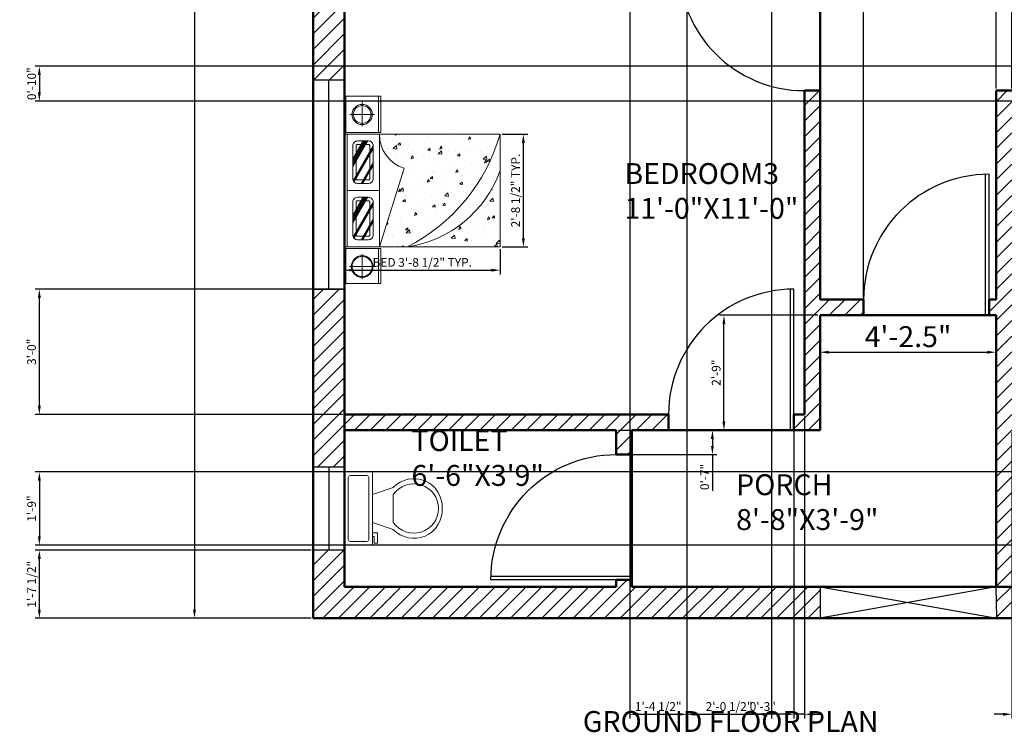
# Model space of a CAD drawing. Units: inches. Extents: x 3064 to 3516, y 2736 to 3280.
# Tile 1 of 5: x 3064 to 3346, y 2736 to 2941. Entities that reach past the tile are written whole.
import ezdxf

# ---------------------------------------------------------------- set-up
doc = ezdxf.new("R2010")
doc.units = ezdxf.units.IN
for name, color, linetype, lineweight in [('A-ANNO-DIMS', 2, 'Continuous', 18), ('A-ANNO-TEXT', 7, 'Continuous', 25), ('A-AREA-IDEN', 6, 'Continuous', 25), ('A-DOOR', 3, 'Continuous', 25), ('A-FLOR-ENTR', 1, 'Continuous', 25), ('A-FLOR-FIXT', 9, 'Continuous', 20), ('A-FURN', 8, 'Continuous', 18), ('A-FURN-PATT', 9, 'Continuous', 13), ('A-GLAZ', 5, 'Continuous', 25), ('A-WALL', 7, 'Continuous', 50), ('A-WALL-PATT', 8, 'Continuous', 13)]:
    doc.layers.add(name, color=color, linetype=linetype, lineweight=lineweight)
doc.styles.get("Standard").update_dxf_attribs({"font": 'arial.ttf'})
doc.dimstyles.new('ISO-25', dxfattribs={"dimtxt": 2.5, "dimasz": 2.5, "dimexe": 1.25, "dimexo": 0.625, "dimtad": 1, "dimlunit": 3, "dimtxsty": 'Standard', "dimcen": 2.5, "dimadec": 0, "dimazin": 0, "dimtfac": 1, "dimtmove": 0, "dimatfit": 3, "dimfxl": 1, "dimarcsym": 0})

# ---------------------------------------------------------------- blocks, each defined once
blk = doc.blocks.new('*D2')
at = {"layer": 'A-ANNO-DIMS', "color": 0, "lineweight": -2, "transparency": 16777216}
for p, q in [((3293.4, 2848.4), (3293.4, 2844.15)), ((3343.9, 2848.4), (3343.9, 2844.15)), ((3295.9, 2845.4), (3341.4, 2845.4))]:
    blk.add_line(p, q, dxfattribs=at)
at = {"layer": 'A-ANNO-DIMS', "color": 0, "transparency": 16777216}
for points in [[(3295.9, 2845.82), (3295.9, 2844.98), (3293.4, 2845.4)], [(3341.4, 2845.82), (3341.4, 2844.98), (3343.9, 2845.4)]]:
    blk.add_solid(points, dxfattribs=at)
at = {"layer": 'Defpoints', "color": 0, "transparency": 16777216}
for p in [(3293.4, 2849.02), (3343.9, 2849.02), (3343.9, 2845.4)]:
    blk.add_point(p, dxfattribs=at)
at = {"layer": 'A-ANNO-DIMS', "color": 0, "transparency": 16777216, "insert": (3318.65, 2849.09), "char_height": 6, "attachment_point": 5}
blk.add_mtext('4\'-2.5"', dxfattribs=at)
blk = doc.blocks.new('*D4')
at = {"layer": 'A-ANNO-DIMS', "color": 0, "lineweight": -2, "transparency": 16777216}
for p, q in [((3147.27, 3211.51), (3112.57, 3211.51)), ((3113.82, 3209.01), (3113.82, 2771.51)), ((3147.27, 2769.01), (3112.57, 2769.01))]:
    blk.add_line(p, q, dxfattribs=at)
at = {"layer": 'A-ANNO-DIMS', "color": 0, "transparency": 16777216}
for points in [[(3113.4, 3209.01), (3114.23, 3209.01), (3113.82, 3211.51)], [(3113.4, 2771.51), (3114.23, 2771.51), (3113.82, 2769.01)]]:
    blk.add_solid(points, dxfattribs=at)
at = {"layer": 'Defpoints', "color": 0, "transparency": 16777216}
for p in [(3147.9, 3211.51), (3113.82, 2769.01), (3147.9, 2769.01)]:
    blk.add_point(p, dxfattribs=at)
at = {"layer": 'A-ANNO-DIMS', "color": 0, "transparency": 16777216, "insert": (3110.13, 2990.26), "char_height": 6, "attachment_point": 5, "rotation": 90}
blk.add_mtext('36\'-10.5"', dxfattribs=at)
blk = doc.blocks.new('*U6')
for p, q in [((9.5, -6), (9.5, -2)), ((-8, -8.5), (-8, -8)), ((-7, -8), (-7, -9.5)), ((-4, -8), (-6, -14)), ((4, -8), (6, -14)), ((-10, -8.5), (-8, -8.5)), ((-10, -9.5), (-10, -8.5)), ((-7, -9.5), (-10, -9.5)), ((4, -14), (-4, -14))]:
    blk.add_line(p, q)
blk.add_lwpolyline([(10.5, -8), (10.5, 0), (-10.5, 0), (-10.5, -8)], close=True)
for points in [[(-9.5, -2), (-9.5, -6)], [(8.5, -1), (-8.5, -1)], [(-8.5, -7), (8.5, -7)]]:
    blk.add_lwpolyline(points)
for centre, radius, start, end in [((-8.625, -1.875), 0.8839, 81.8699, 188.1301), ((8.625, -1.875), 0.8839, 351.8699, 98.1301), ((-8.625, -6.125), 0.8839, 171.869898, 278.1301), ((8.625, -6.125), 0.8839, 261.8699, 8.1301), ((-0.4772, -19.9188), 8.0953, 133.01722, 273.38), ((0.0374, -19.8731), 7.127, 124.50543, 269.7), ((-0.0373, -19.8731), 7.127, 270.3, 55.4946), ((0.4773, -19.9188), 8.0953, 266.62, 46.9828)]:
    blk.add_arc(centre, radius, start, end)
blk = doc.blocks.new('DOOR-SWING-36IN')
for p, q in [((-1, -4.5), (-1, 36)), ((0, 0), (0, 36))]:
    blk.add_line(p, q)
blk.add_arc((0, 0), 36, 90, 180)
blk = doc.blocks.new('WIN-60IN')
for p, q in [((0, 60), (0, 0)), ((9, 60), (0, 60)), ((4.5, 60), (4.5, 0)), ((9, 0), (9, 60)), ((0, 0), (9, 0))]:
    blk.add_line(p, q)
blk = doc.blocks.new('WIN-24IN')
for p, q in [((0, 24), (9, 24)), ((0, 0), (0, 24)), ((4.5, 24), (4.5, 0)), ((9, 24), (9, 0)), ((9, 0), (0, 0))]:
    blk.add_line(p, q)
blk = doc.blocks.new('BEDSIDE-TABLE-A')
for p, q in [((0, 0), (0, 10.49)), ((0, 10.49), (10.04, 10.49)), ((4.67, 1.81), (4.67, 8.9)), ((9.38, 0), (9.38, 10.49)), ((10.04, 10.49), (10.04, 0)), ((1.1, 5.18), (8.23, 5.18)), ((10.04, 0), (0, 0))]:
    blk.add_line(p, q)
for radius in [2.89, 2.54]:
    blk.add_circle((4.67, 5.18), radius)
blk = doc.blocks.new('BEDSIDE-TABLE-B')
for p, q in [((10.04, 10.04), (0, 10.04)), ((0, 10.04), (0, 0)), ((9.34, 0), (9.34, 10.04)), ((10.04, 0), (10.04, 10.04)), ((4.67, 1.21), (4.67, 8.43)), ((1.04, 4.86), (8.55, 4.86)), ((0, 0), (10.04, 0))]:
    blk.add_line(p, q)
for radius in [3.11, 2.89]:
    blk.add_circle((4.67, 4.86), radius)
blk = doc.blocks.new('BED-FRAME-AND-COVER')
for p, q in [((0, 32.36), (44.63, 32.36)), ((0, 0), (0, 32.36)), ((0.73, 0), (0.73, 32.36)), ((10.02, 0), (10.02, 32.36)), ((44.63, 32.36), (44.63, 0)), ((10.02, 0), (17.09, 22.61)), ((10.02, 16.18), (0.73, 16.18)), ((44.63, 0), (0, 0))]:
    blk.add_line(p, q)
for centre, radius, start, end in [((20, 32.16), 9.98, 178.8468, 253.0453), ((-5.57, 46.57), 52.17, 296.7955, 344.1914), ((13.16, 33.03), 33.38, 278.2583, 340.5572)]:
    blk.add_arc(centre, radius, start, end)
blk = doc.blocks.new('*D29')
at = {"layer": 'A-ANNO-DIMS', "color": 0, "lineweight": -2, "transparency": 16777216}
for p, q in [((3156.9, 2875.02), (3156.9, 2867.7)), ((3201.53, 2875.02), (3201.53, 2867.7)), ((3159.4, 2868.95), (3199.03, 2868.95))]:
    blk.add_line(p, q, dxfattribs=at)
at = {"layer": 'A-ANNO-DIMS', "color": 0, "transparency": 16777216}
for points in [[(3159.4, 2869.37), (3159.4, 2868.54), (3156.9, 2868.95)], [(3199.03, 2869.37), (3199.03, 2868.54), (3201.53, 2868.95)]]:
    blk.add_solid(points, dxfattribs=at)
at = {"layer": 'Defpoints', "color": 0, "transparency": 16777216}
for p in [(3156.9, 2875.65), (3201.53, 2875.65), (3201.53, 2868.95)]:
    blk.add_point(p, dxfattribs=at)
at = {"layer": 'A-ANNO-DIMS', "color": 0, "transparency": 16777216, "insert": (3179.21, 2870.87), "char_height": 2.5, "attachment_point": 5}
blk.add_mtext('BED 3\'-8 1/2" TYP.', dxfattribs=at)
blk = doc.blocks.new('*D30')
at = {"layer": 'A-ANNO-DIMS', "color": 0, "lineweight": -2, "transparency": 16777216}
for p, q in [((3202.15, 2908.01), (3209.47, 2908.01)), ((3208.22, 2878.15), (3208.22, 2905.51)), ((3202.15, 2875.65), (3209.47, 2875.65))]:
    blk.add_line(p, q, dxfattribs=at)
at = {"layer": 'A-ANNO-DIMS', "color": 0, "transparency": 16777216}
for points in [[(3207.81, 2905.51), (3208.64, 2905.51), (3208.22, 2908.01)], [(3207.81, 2878.15), (3208.64, 2878.15), (3208.22, 2875.65)]]:
    blk.add_solid(points, dxfattribs=at)
at = {"layer": 'Defpoints', "color": 0, "transparency": 16777216}
for p in [(3201.53, 2908.01), (3208.22, 2908.01), (3201.53, 2875.65)]:
    blk.add_point(p, dxfattribs=at)
at = {"layer": 'A-ANNO-DIMS', "color": 0, "transparency": 16777216, "insert": (3206.31, 2891.83), "char_height": 2.5, "attachment_point": 5, "rotation": 90}
blk.add_mtext('2\'-8 1/2" TYP.', dxfattribs=at)
blk = doc.blocks.new('*D37')
at = {"layer": 'A-ANNO-DIMS', "color": 0, "lineweight": -2, "transparency": 16777216}
for p, q in [((3147.27, 2788.51), (3068.05, 2788.51)), ((3069.3, 2771.51), (3069.3, 2786.01)), ((3147.27, 2769.01), (3068.05, 2769.01))]:
    blk.add_line(p, q, dxfattribs=at)
at = {"layer": 'A-ANNO-DIMS', "color": 0, "transparency": 16777216}
for points in [[(3068.88, 2786.01), (3069.71, 2786.01), (3069.3, 2788.51)], [(3068.88, 2771.51), (3069.71, 2771.51), (3069.3, 2769.01)]]:
    blk.add_solid(points, dxfattribs=at)
at = {"layer": 'Defpoints', "color": 0, "transparency": 16777216}
for p in [(3069.3, 2788.51), (3147.9, 2788.51), (3147.9, 2769.01)]:
    blk.add_point(p, dxfattribs=at)
at = {"layer": 'A-ANNO-DIMS', "color": 0, "transparency": 16777216, "insert": (3067.38, 2778.76), "char_height": 2.5, "attachment_point": 5, "rotation": 90}
blk.add_mtext('1\'-7 1/2"', dxfattribs=at)
blk = doc.blocks.new('*D38')
at = {"layer": 'A-ANNO-DIMS', "color": 0, "lineweight": -2, "transparency": 16777216}
for p, q in [((3156.27, 2863.51), (3068.05, 2863.51)), ((3069.3, 2830.01), (3069.3, 2861.01)), ((3156.27, 2827.51), (3068.05, 2827.51))]:
    blk.add_line(p, q, dxfattribs=at)
at = {"layer": 'A-ANNO-DIMS', "color": 0, "transparency": 16777216}
for points in [[(3068.88, 2861.01), (3069.71, 2861.01), (3069.3, 2863.51)], [(3068.88, 2830.01), (3069.71, 2830.01), (3069.3, 2827.51)]]:
    blk.add_solid(points, dxfattribs=at)
at = {"layer": 'Defpoints', "color": 0, "transparency": 16777216}
for p in [(3069.3, 2863.51), (3156.9, 2863.51), (3156.9, 2827.51)]:
    blk.add_point(p, dxfattribs=at)
at = {"layer": 'A-ANNO-DIMS', "color": 0, "transparency": 16777216, "insert": (3067.39, 2845.51), "char_height": 2.5, "attachment_point": 5, "rotation": 90}
blk.add_mtext('3\'-0"', dxfattribs=at)
blk = doc.blocks.new('*D44')
at = {"layer": 'A-ANNO-DIMS', "color": 0, "lineweight": -2, "transparency": 16777216}
for p, q in [((3341.4, 3239.11), (3325.18, 3239.11)), ((3343.9, 2921.14), (3343.9, 3240.36)), ((3348.4, 3239.11), (3343.9, 3239.11)), ((3348.4, 2921.14), (3348.4, 3240.36)), ((3350.9, 3239.11), (3353.4, 3239.11))]:
    blk.add_line(p, q, dxfattribs=at)
at = {"layer": 'A-ANNO-DIMS', "color": 0, "transparency": 16777216}
for points in [[(3341.4, 3239.53), (3341.4, 3238.7), (3343.9, 3239.11)], [(3350.9, 3239.53), (3350.9, 3238.7), (3348.4, 3239.11)]]:
    blk.add_solid(points, dxfattribs=at)
at = {"layer": 'Defpoints', "color": 0, "transparency": 16777216}
for p in [(3343.9, 3239.11), (3343.9, 2920.51), (3348.4, 2920.51)]:
    blk.add_point(p, dxfattribs=at)
at = {"layer": 'A-ANNO-DIMS', "color": 0, "transparency": 16777216, "insert": (3332.04, 3241.03), "char_height": 2.5, "attachment_point": 5}
blk.add_mtext('0\'-4 1/2"', dxfattribs=at)
blk = doc.blocks.new('*D45')
at = {"layer": 'A-ANNO-DIMS', "color": 0, "lineweight": -2, "transparency": 16777216}
for p, q in [((3386.77, 2927.51), (3068.05, 2927.51)), ((3069.3, 2925.01), (3069.3, 2920.01)), ((3386.77, 2917.51), (3068.05, 2917.51))]:
    blk.add_line(p, q, dxfattribs=at)
at = {"layer": 'A-ANNO-DIMS', "color": 0, "transparency": 16777216}
for points in [[(3068.88, 2925.01), (3069.71, 2925.01), (3069.3, 2927.51)], [(3068.88, 2920.01), (3069.71, 2920.01), (3069.3, 2917.51)]]:
    blk.add_solid(points, dxfattribs=at)
at = {"layer": 'Defpoints', "color": 0, "transparency": 16777216}
for p in [(3387.4, 2927.51), (3069.3, 2917.51), (3387.4, 2917.51)]:
    blk.add_point(p, dxfattribs=at)
at = {"layer": 'A-ANNO-DIMS', "color": 0, "transparency": 16777216, "insert": (3067.4, 2922.51), "char_height": 2.5, "attachment_point": 5, "rotation": 90}
blk.add_mtext('0\'-10"', dxfattribs=at)
blk = doc.blocks.new('*D47')
at = {"layer": 'A-ANNO-DIMS', "color": 0, "lineweight": -2, "transparency": 16777216}
for p, q in [((3292.77, 2856.01), (3264.55, 2856.01)), ((3265.8, 2825.51), (3265.8, 2853.51)), ((3292.77, 2823.01), (3264.55, 2823.01))]:
    blk.add_line(p, q, dxfattribs=at)
at = {"layer": 'A-ANNO-DIMS', "color": 0, "transparency": 16777216}
for points in [[(3265.38, 2853.51), (3266.21, 2853.51), (3265.8, 2856.01)], [(3265.38, 2825.51), (3266.21, 2825.51), (3265.8, 2823.01)]]:
    blk.add_solid(points, dxfattribs=at)
at = {"layer": 'Defpoints', "color": 0, "transparency": 16777216}
for p in [(3265.8, 2856.01), (3293.4, 2856.01), (3293.4, 2823.01)]:
    blk.add_point(p, dxfattribs=at)
at = {"layer": 'A-ANNO-DIMS', "color": 0, "transparency": 16777216, "insert": (3263.9, 2839.51), "char_height": 2.5, "attachment_point": 5, "rotation": 90}
blk.add_mtext('2\'-9"', dxfattribs=at)
blk = doc.blocks.new('*D48')
at = {"layer": 'A-ANNO-DIMS', "color": 0, "lineweight": -2, "transparency": 16777216}
for p, q in [((3417.77, 2811.01), (3068.05, 2811.01)), ((3069.3, 2808.51), (3069.3, 2792.51)), ((3417.77, 2790.01), (3068.05, 2790.01))]:
    blk.add_line(p, q, dxfattribs=at)
at = {"layer": 'A-ANNO-DIMS', "color": 0, "transparency": 16777216}
for points in [[(3068.88, 2808.51), (3069.71, 2808.51), (3069.3, 2811.01)], [(3068.88, 2792.51), (3069.71, 2792.51), (3069.3, 2790.01)]]:
    blk.add_solid(points, dxfattribs=at)
at = {"layer": 'Defpoints', "color": 0, "transparency": 16777216}
for p in [(3418.4, 2811.01), (3069.3, 2790.01), (3418.4, 2790.01)]:
    blk.add_point(p, dxfattribs=at)
at = {"layer": 'A-ANNO-DIMS', "color": 0, "transparency": 16777216, "insert": (3067.4, 2800.51), "char_height": 2.5, "attachment_point": 5, "rotation": 90}
blk.add_mtext('1\'-9"', dxfattribs=at)
blk = doc.blocks.new('*D53')
at = {"layer": 'A-ANNO-DIMS', "color": 0, "lineweight": -2, "transparency": 16777216}
for p, q in [((3238.74, 2963.39), (3238.74, 2740.16)), ((3255.12, 2963.39), (3255.12, 2740.16)), ((3241.24, 2741.41), (3252.62, 2741.41))]:
    blk.add_line(p, q, dxfattribs=at)
at = {"layer": 'A-ANNO-DIMS', "color": 0, "transparency": 16777216}
for points in [[(3241.24, 2741.83), (3241.24, 2741), (3238.74, 2741.41)], [(3252.62, 2741.83), (3252.62, 2741), (3255.12, 2741.41)]]:
    blk.add_solid(points, dxfattribs=at)
at = {"layer": 'Defpoints', "color": 0, "transparency": 16777216}
for p in [(3238.74, 2964.01), (3255.12, 2964.01), (3255.12, 2741.41)]:
    blk.add_point(p, dxfattribs=at)
at = {"layer": 'A-ANNO-DIMS', "color": 0, "transparency": 16777216, "insert": (3246.93, 2743.33), "char_height": 2.5, "attachment_point": 5}
blk.add_mtext('1\'-4 1/2"', dxfattribs=at)
blk = doc.blocks.new('*D54')
at = {"layer": 'A-ANNO-DIMS', "color": 0, "lineweight": -2, "transparency": 16777216}
for p, q in [((3255.12, 2963.39), (3255.12, 2740.16)), ((3279.41, 2963.39), (3279.41, 2740.16)), ((3257.62, 2741.41), (3276.91, 2741.41))]:
    blk.add_line(p, q, dxfattribs=at)
at = {"layer": 'A-ANNO-DIMS', "color": 0, "transparency": 16777216}
for points in [[(3257.62, 2741.83), (3257.62, 2741), (3255.12, 2741.41)], [(3276.91, 2741.83), (3276.91, 2741), (3279.41, 2741.41)]]:
    blk.add_solid(points, dxfattribs=at)
at = {"layer": 'Defpoints', "color": 0, "transparency": 16777216}
for p in [(3255.12, 2964.01), (3279.41, 2964.01), (3279.41, 2741.41)]:
    blk.add_point(p, dxfattribs=at)
at = {"layer": 'A-ANNO-DIMS', "color": 0, "transparency": 16777216, "insert": (3267.26, 2743.33), "char_height": 2.5, "attachment_point": 5}
blk.add_mtext('2\'-0 1/2"', dxfattribs=at)
blk = doc.blocks.new('*D58')
at = {"layer": 'A-ANNO-DIMS', "color": 0, "lineweight": -2, "transparency": 16777216}
for p, q in [((3235.52, 2823.01), (3263.75, 2823.01)), ((3262.5, 2820.51), (3262.5, 2818.51)), ((3235.52, 2816.01), (3263.75, 2816.01)), ((3262.5, 2816.01), (3262.5, 2805.62))]:
    blk.add_line(p, q, dxfattribs=at)
at = {"layer": 'A-ANNO-DIMS', "color": 0, "transparency": 16777216}
for points in [[(3262.08, 2820.51), (3262.91, 2820.51), (3262.5, 2823.01)], [(3262.08, 2818.51), (3262.91, 2818.51), (3262.5, 2816.01)]]:
    blk.add_solid(points, dxfattribs=at)
at = {"layer": 'Defpoints', "color": 0, "transparency": 16777216}
for p in [(3234.9, 2823.01), (3234.9, 2816.01), (3262.5, 2816.01)]:
    blk.add_point(p, dxfattribs=at)
at = {"layer": 'A-ANNO-DIMS', "color": 0, "transparency": 16777216, "insert": (3260.6, 2809.57), "char_height": 2.5, "attachment_point": 5, "rotation": 90}
blk.add_mtext('0\'-7"', dxfattribs=at)
blk = doc.blocks.new('*D60')
at = {"layer": 'A-ANNO-DIMS', "color": 0, "lineweight": -2, "transparency": 16777216}
for p, q in [((3285.9, 2826.89), (3285.9, 2740.16)), ((3288.9, 2826.89), (3288.9, 2740.16)), ((3283.4, 2741.41), (3273, 2741.41)), ((3288.9, 2741.41), (3285.9, 2741.41)), ((3291.4, 2741.41), (3293.9, 2741.41))]:
    blk.add_line(p, q, dxfattribs=at)
at = {"layer": 'A-ANNO-DIMS', "color": 0, "transparency": 16777216}
for points in [[(3283.4, 2741.83), (3283.4, 2741), (3285.9, 2741.41)], [(3291.4, 2741.83), (3291.4, 2741), (3288.9, 2741.41)]]:
    blk.add_solid(points, dxfattribs=at)
at = {"layer": 'Defpoints', "color": 0, "transparency": 16777216}
for p in [(3285.9, 2827.51), (3288.9, 2827.51), (3285.9, 2741.41)]:
    blk.add_point(p, dxfattribs=at)
at = {"layer": 'A-ANNO-DIMS', "color": 0, "transparency": 16777216, "insert": (3276.95, 2743.32), "char_height": 2.5, "attachment_point": 5}
blk.add_mtext('0\'-3"', dxfattribs=at)
blk = doc.blocks.new('*D61')
at = {"layer": 'A-ANNO-DIMS', "color": 0, "lineweight": -2, "transparency": 16777216}
for p, q in [((3293.4, 2861.14), (3293.4, 3240.36)), ((3295.9, 3239.11), (3303.4, 3239.11)), ((3305.9, 2861.14), (3305.9, 3240.36)), ((3305.9, 3239.11), (3321.88, 3239.11))]:
    blk.add_line(p, q, dxfattribs=at)
at = {"layer": 'A-ANNO-DIMS', "color": 0, "transparency": 16777216}
for points in [[(3295.9, 3239.53), (3295.9, 3238.7), (3293.4, 3239.11)], [(3303.4, 3239.53), (3303.4, 3238.7), (3305.9, 3239.11)]]:
    blk.add_solid(points, dxfattribs=at)
at = {"layer": 'Defpoints', "color": 0, "transparency": 16777216}
for p in [(3305.9, 3239.11), (3293.4, 2860.51), (3305.9, 2860.51)]:
    blk.add_point(p, dxfattribs=at)
at = {"layer": 'A-ANNO-DIMS', "color": 0, "transparency": 16777216, "insert": (3315.14, 3241.03), "char_height": 2.5, "attachment_point": 5}
blk.add_mtext('1\'-0 1/2"', dxfattribs=at)
blk = doc.blocks.new('*D63')
at = {"layer": 'A-ANNO-DIMS', "color": 0, "lineweight": -2, "transparency": 16777216}
for p, q in [((3348.4, 2822.39), (3348.4, 2740.16)), ((3350.4, 2822.39), (3350.4, 2740.16)), ((3345.9, 2741.41), (3343.4, 2741.41)), ((3348.4, 2741.41), (3350.4, 2741.41)), ((3352.9, 2741.41), (3363.29, 2741.41))]:
    blk.add_line(p, q, dxfattribs=at)
at = {"layer": 'A-ANNO-DIMS', "color": 0, "transparency": 16777216}
for points in [[(3345.9, 2741.83), (3345.9, 2741), (3348.4, 2741.41)], [(3352.9, 2741.83), (3352.9, 2741), (3350.4, 2741.41)]]:
    blk.add_solid(points, dxfattribs=at)
at = {"layer": 'Defpoints', "color": 0, "transparency": 16777216}
for p in [(3348.4, 2823.01), (3350.4, 2823.01), (3350.4, 2741.41)]:
    blk.add_point(p, dxfattribs=at)
at = {"layer": 'A-ANNO-DIMS', "color": 0, "transparency": 16777216, "insert": (3359.35, 2743.32), "char_height": 2.5, "attachment_point": 5}
blk.add_mtext('0\'-2"', dxfattribs=at)

msp = doc.modelspace()

# ---------------------------------------------------------------- hatches: boundary and pattern name
at = {"layer": 'A-FURN-PATT'}
h = msp.add_hatch(dxfattribs=at)
h.set_pattern_fill('ANSI31', color=256, scale=0.070287317, angle=15.041628, style=0)
h.paths.add_polyline_path([(3159.249, 2898.533), (3159.249, 2898.613), (3159.249, 2899.06), (3159.249, 2899.507), (3159.249, 2899.587), (3162.981, 2906.063), (3163.028, 2906.063), (3163.285, 2906.063), (3163.543, 2906.063), (3163.589, 2906.063)])
h = msp.add_hatch(dxfattribs=at)
h.set_pattern_fill('ANSI31', color=256, scale=0.070284384, angle=15.041628, style=0)
h.paths.add_polyline_path([(3159.249, 2899.981), (3159.249, 2900.062), (3159.249, 2900.508), (3159.249, 2900.955), (3159.249, 2901.036), (3162.147, 2906.063), (3162.193, 2906.063), (3162.451, 2906.063), (3162.708, 2906.063), (3162.754, 2906.063)])
h = msp.add_hatch(dxfattribs=at)
h.set_pattern_fill('AR-CONC', color=256, scale=0.044631, angle=450, style=0)
h.set_pattern_definition([(220, (5689.692, 3289.2617), (0.711375, -8.131058), [0.850218, -9.352396]), (275, (5689.692, 3289.262), (-8.527021, 1.572917), [0.680174, -7.481917]), (169.549, (5689.7516, 3288.584), (-7.815608, -6.55817), [0.722574, -7.94831]), (223.8158, (5687.425, 3289.262), (1.876385, -12.09849), [1.275327, -14.028594]), (173.3644, (5687.581, 3288.253), (-11.042814, -10.595554), [1.08386, -11.922464]), (278.816, (5687.425, 3289.262), (-11.042795, -10.59557), [1.02026, -11.222875]), (249, (5687.992, 3288.128), (4.564198, -6.766702), [0.850218, -9.352396]), (304, (5687.992, 3288.128), (-8.220467, -2.758277), [0.680174, -7.481917]), (198.5486, (5688.372, 3287.564), (-3.656287, -9.52496), [0.722574, -7.94831]), (232.5, (5689.6923, 3289.2617), (-3.7737637, -0.137847), [0, -7.391227, 0, -7.595279, 0, -7.510257]), (262.5, (5689.6923, 3289.2617), (-4.471145, -2.982219), [0, -4.330443, 0, -7.221183, 0, -2.8624]), (302.5, (5689.6923, 3291.7896), (0.2556787, -6.0515243), [0, -2.834059, 0, -8.842265, 0, -11.733006]), (312.5, (5689.6923, 3292.9233), (-1.134806, -6.611132), [0, -3.684277, 0, -5.872171, 0, -8.332134])])
edge = h.paths.add_edge_path()
edge.add_ellipse((3176.893, 2907.806), major_axis=(7.055, 7.055), ratio=1, start_angle=136.15316, end_angle=208.04534, ccw=False)
edge.add_line((3166.918, 2907.605), (3166.918, 2908.007))
edge.add_line((3166.918, 2908.007), (3201.528, 2908.007))
edge.add_ellipse((3151.329, 2922.22), major_axis=(36.892, 36.892), ratio=1, start_angle=251.7955, end_angle=299.1914, ccw=False)
edge.add_line((3174.849, 2875.649), (3166.918, 2875.649))
edge.add_line((3166.918, 2875.649), (3173.983, 2898.262))
edge = h.paths.add_edge_path()
edge.add_line((3201.528, 2897.57), (3201.528, 2875.649))
edge.add_line((3201.528, 2875.649), (3174.849, 2875.649))
edge.add_ellipse((3170.054, 2908.68), major_axis=(23.601, -23.601), ratio=1, start_angle=323.25827, end_angle=385.55722)
h = msp.add_hatch(dxfattribs=at)
h.set_pattern_fill('ANSI31', color=256, scale=0.070289157, angle=15.041628, style=0)
h.paths.add_polyline_path([(3159.656, 2894.255), (3159.629, 2894.288), (3159.478, 2894.474), (3159.353, 2894.704), (3159.331, 2894.746), (3165.137, 2904.819), (3165.137, 2904.738), (3165.137, 2904.291), (3165.137, 2903.845), (3165.137, 2903.764)])
h = msp.add_hatch(dxfattribs=at)
h.set_pattern_fill('ANSI31', color=256, scale=0.070287466, angle=15.041628, style=0)
h.paths.add_polyline_path([(3162.239, 2893.884), (3162.193, 2893.884), (3161.935, 2893.884), (3161.678, 2893.884), (3161.631, 2893.884), (3165.137, 2899.965), (3165.137, 2899.885), (3165.137, 2899.438), (3165.137, 2898.991), (3165.137, 2898.911)])
h = msp.add_hatch(dxfattribs=at)
h.set_pattern_fill('ANSI31', color=256, scale=0.070289772, angle=15.041628, style=0)
h.paths.add_polyline_path([(3159.249, 2882.354), (3159.249, 2882.435), (3159.249, 2882.881), (3159.249, 2883.328), (3159.249, 2883.409), (3162.981, 2889.884), (3163.028, 2889.884), (3163.285, 2889.884), (3163.543, 2889.884), (3163.589, 2889.884)])
h = msp.add_hatch(dxfattribs=at)
h.set_pattern_fill('ANSI31', color=256, scale=0.070286859, angle=15.041628, style=0)
h.paths.add_polyline_path([(3159.249, 2883.802), (3159.249, 2883.883), (3159.249, 2884.33), (3159.249, 2884.777), (3159.249, 2884.857), (3162.147, 2889.884), (3162.193, 2889.884), (3162.451, 2889.884), (3162.708, 2889.884), (3162.754, 2889.884)])
h = msp.add_hatch(dxfattribs=at)
h.set_pattern_fill('ANSI31', color=256, scale=0.070279531, angle=15.041628, style=0)
h.paths.add_polyline_path([(3159.656, 2878.076), (3159.629, 2878.11), (3159.478, 2878.295), (3159.353, 2878.526), (3159.331, 2878.567), (3165.137, 2888.64), (3165.137, 2888.559), (3165.137, 2888.113), (3165.137, 2887.666), (3165.137, 2887.585)])
h = msp.add_hatch(dxfattribs=at)
h.set_pattern_fill('ANSI31', color=256, scale=0.070289911, angle=15.041628, style=0)
h.paths.add_polyline_path([(3162.239, 2877.705), (3162.193, 2877.705), (3161.935, 2877.705), (3161.678, 2877.705), (3161.631, 2877.705), (3165.137, 2883.786), (3165.137, 2883.706), (3165.137, 2883.259), (3165.137, 2882.812), (3165.137, 2882.732)])
at = {"layer": 'A-WALL-PATT'}
h = msp.add_hatch(dxfattribs=at)
h.set_pattern_fill('ANSI31', color=256)
h.paths.add_polyline_path([(3156.897, 2985.015), (3147.897, 2985.015), (3147.897, 2923.515), (3156.897, 2923.515)])
h.paths.add_polyline_path([(3156.897, 2863.515), (3147.897, 2863.515), (3147.897, 2812.515), (3156.897, 2812.515)])
h.paths.add_polyline_path([(3293.397, 2778.015), (3239.397, 2778.015), (3239.397, 2780.015), (3234.897, 2780.015), (3234.897, 2778.015), (3156.897, 2778.015), (3156.897, 2788.515), (3147.897, 2788.515), (3147.897, 2769.015), (3293.397, 2769.015)])
h.paths.add_polyline_path([(3369.397, 2778.015), (3343.897, 2778.015), (3344.15, 2769.015), (3369.397, 2769.015)])
h.paths.add_polyline_path([(3435.397, 2788.515), (3426.397, 2788.515), (3426.397, 2778.015), (3405.397, 2778.015), (3405.397, 2769.015), (3435.397, 2769.015)])
h.paths.add_polyline_path([(3435.397, 2960.265), (3426.397, 2960.265), (3426.397, 2812.515), (3435.397, 2812.515)])
h.paths.add_polyline_path([(3435.397, 3094.515), (3426.397, 3094.515), (3426.397, 3020.265), (3435.397, 3020.265)])
h.paths.add_polyline_path([(3435.397, 3211.515), (3147.897, 3211.515), (3147.897, 3154.515), (3156.897, 3154.515), (3156.897, 3202.515), (3426.397, 3202.515), (3426.397, 3154.515), (3435.397, 3154.515)])
h.paths.add_polyline_path([(3293.397, 3202.515), (3288.897, 3202.515), (3288.897, 3046.515), (3285.897, 3046.515), (3285.897, 3042.015), (3296.397, 3042.015), (3296.397, 3046.515), (3293.397, 3046.515)])
h.paths.add_polyline_path([(3426.397, 3046.515), (3332.397, 3046.515), (3332.397, 3042.015), (3426.397, 3042.015)])
h.paths.add_polyline_path([(3249.897, 3046.515), (3156.897, 3046.515), (3156.897, 3042.015), (3249.897, 3042.015)])
h.paths.add_polyline_path([(3156.897, 3094.515), (3147.897, 3094.515), (3147.897, 3021.015), (3156.897, 3021.015)])
h.paths.add_polyline_path([(3293.397, 2964.015), (3156.897, 2964.015), (3156.897, 2959.515), (3288.897, 2959.515), (3288.897, 2956.515), (3293.397, 2956.515)])
h.paths.add_polyline_path([(3249.897, 2827.515), (3156.897, 2827.515), (3156.897, 2823.015), (3234.897, 2823.015), (3234.897, 2816.015), (3239.397, 2816.015), (3239.397, 2823.015), (3249.897, 2823.015)])
h.paths.add_polyline_path([(3293.397, 2920.515), (3288.897, 2920.515), (3288.897, 2827.515), (3285.897, 2827.515), (3285.897, 2823.015), (3293.397, 2823.015), (3293.397, 2856.015), (3305.897, 2856.015), (3305.897, 2860.515), (3293.397, 2860.515)])
h.paths.add_polyline_path([(3348.397, 2920.515), (3343.897, 2920.515), (3343.897, 2860.515), (3341.897, 2860.515), (3341.897, 2856.015), (3343.897, 2856.015), (3343.897, 2778.015), (3348.397, 2778.015), (3348.397, 2823.015), (3350.397, 2823.015), (3350.397, 2827.515), (3348.397, 2827.515)])
h.paths.add_polyline_path([(3426.397, 2827.515), (3386.397, 2827.515), (3386.397, 2823.015), (3426.397, 2823.015)])

# ---------------------------------------------------------------- linework, layer by layer
at = {"layer": 'A-FLOR-ENTR'}
for p, q in [((3293.397, 2778.015), (3293.397, 2769.015)), ((3343.897, 2778.015), (3293.397, 2778.015)), ((3293.397, 2778.015), (3344.15, 2769.015)), ((3343.897, 2778.015), (3293.397, 2769.015)), ((3344.15, 2769.015), (3343.897, 2778.015)), ((3293.397, 2769.015), (3344.15, 2769.015))]:
    msp.add_line(p, q, dxfattribs=at)
at = {"layer": 'A-FURN'}
for points in [[(3159.249, 2904.724), (3159.249, 2895.223, 0.4142136), (3160.588, 2893.884), (3163.798, 2893.884, 0.4142136), (3165.137, 2895.223), (3165.137, 2904.724, 0.4142136), (3163.798, 2906.063), (3160.588, 2906.063, 0.4142136)], [(3160.253, 2904.724), (3160.253, 2895.223, 0.4142136), (3160.588, 2894.888), (3163.798, 2894.888, 0.4142136), (3164.133, 2895.223), (3164.133, 2904.724, 0.4142136), (3163.798, 2905.059), (3160.588, 2905.059, 0.4142136)], [(3159.249, 2888.545), (3159.249, 2879.044, 0.4142136), (3160.588, 2877.705), (3163.798, 2877.705, 0.4142136), (3165.137, 2879.044), (3165.137, 2888.545, 0.4142136), (3163.798, 2889.884), (3160.588, 2889.884, 0.4142136)], [(3160.253, 2888.545), (3160.253, 2879.044, 0.4142136), (3160.588, 2878.709), (3163.798, 2878.709, 0.4142136), (3164.133, 2879.044), (3164.133, 2888.545, 0.4142136), (3163.798, 2888.88), (3160.588, 2888.88, 0.4142136)]]:
    msp.add_lwpolyline(points, format="xyb", close=True, dxfattribs=at)
at = {"layer": 'A-WALL'}
for p, q in [((3147.897, 3211.515), (3147.897, 2769.015)), ((3156.897, 3202.515), (3156.897, 2778.015)), ((3293.397, 2964.015), (3293.397, 2860.515)), ((3293.397, 2920.515), (3288.897, 2920.515)), ((3288.897, 2920.515), (3288.897, 2827.515)), ((3343.897, 2920.515), (3343.897, 2860.515)), ((3343.897, 2920.515), (3348.397, 2920.515)), ((3293.397, 2860.515), (3305.897, 2860.515)), ((3305.897, 2860.515), (3305.897, 2856.015)), ((3341.897, 2856.015), (3341.897, 2860.515)), ((3341.897, 2860.515), (3343.897, 2860.515)), ((3293.397, 2856.015), (3343.897, 2856.015)), ((3293.397, 2856.015), (3293.397, 2823.015)), ((3343.897, 2856.015), (3343.897, 2778.015)), ((3156.897, 2827.515), (3249.897, 2827.515)), ((3156.897, 2827.515), (3249.897, 2827.515)), ((3249.897, 2823.015), (3249.897, 2827.515)), ((3288.897, 2827.515), (3285.897, 2827.515)), ((3285.897, 2827.515), (3285.897, 2823.015)), ((3285.897, 2827.515), (3288.897, 2827.515)), ((3285.897, 2827.515), (3288.897, 2827.515)), ((3156.897, 2823.015), (3234.897, 2823.015)), ((3156.897, 2823.015), (3234.897, 2823.015)), ((3234.897, 2823.015), (3234.897, 2816.015)), ((3239.397, 2823.015), (3239.397, 2778.015)), ((3239.397, 2823.015), (3293.397, 2823.015)), ((3239.397, 2823.015), (3293.397, 2823.015)), ((3285.897, 2823.015), (3249.897, 2823.015)), ((3234.897, 2816.015), (3239.397, 2816.015)), ((3239.397, 2780.015), (3234.897, 2780.015)), ((3234.897, 2780.015), (3234.897, 2778.015)), ((3156.897, 2778.015), (3234.897, 2778.015)), ((3239.397, 2778.015), (3426.397, 2778.015)), ((3147.897, 2769.015), (3435.397, 2769.015))]:
    msp.add_line(p, q, dxfattribs=at)

# ---------------------------------------------------------------- block references
at = {"layer": 'A-DOOR', "rotation": 90.00000000000033}
msp.add_blockref('DOOR-SWING-36IN', (3288.897, 2956.515), dxfattribs=at)
at = {"layer": 'A-DOOR'}
for p in [(3341.897, 2860.515), (3285.897, 2827.515)]:
    msp.add_blockref('DOOR-SWING-36IN', p, dxfattribs=at)
at = {"layer": 'A-DOOR', "extrusion": (0, 0, -1), "zscale": -1, "rotation": 269.9999999999993}
msp.add_blockref('DOOR-SWING-36IN', (-3234.897, 2780.015), dxfattribs=at)
at = {"layer": 'A-FLOR-FIXT', "rotation": 90}
msp.add_blockref('*U6', (3156.897, 2800.515), dxfattribs=at)
at = {"layer": 'A-FURN'}
for name, p in [('BEDSIDE-TABLE-A', (3157.284, 2908.488)), ('BED-FRAME-AND-COVER', (3156.897, 2875.649)), ('BEDSIDE-TABLE-B', (3157.284, 2865.126))]:
    msp.add_blockref(name, p, dxfattribs=at)
at = {"layer": 'A-GLAZ', "rotation": 180}
msp.add_blockref('WIN-60IN', (3156.897, 2923.515), dxfattribs=at)
at = {"layer": 'A-GLAZ'}
msp.add_blockref('WIN-24IN', (3147.897, 2788.515), dxfattribs=at)

# ---------------------------------------------------------------- texts
at = {"layer": 'A-ANNO-TEXT', "insert": (3225.287, 2742.346), "char_height": 6, "attachment_point": 1}
msp.add_mtext_dynamic_manual_height_columns('GROUND FLOOR PLAN', width=115.8357, gutter_width=12.5, heights=[0], dxfattribs=at)
at = {"layer": 'A-AREA-IDEN', "insert": (3237.233, 2899.704), "char_height": 6, "attachment_point": 1}
msp.add_mtext('BEDROOM3\\P11\'-0"X11\'-0"', dxfattribs=at)
at = {"layer": 'A-AREA-IDEN', "char_height": 6, "attachment_point": 1}
for s, width, insert in [('TOILET\\P6\'-6"X3\'9"', 17.38334, (3176.112, 2823.015)), ('PORCH\\P8\'-8"X3\'-9"', 32.19123, (3269.293, 2810.341))]:
    msp.add_mtext_dynamic_manual_height_columns(s, width=width, gutter_width=12.5, heights=[0], dxfattribs=dict(at, insert=insert))

# ---------------------------------------------------------------- dimensions: what is measured, and where the dimension line sits
at = {"layer": 'A-ANNO-DIMS'}
for base, p1, p2, override, picture, middle in [((3305.897, 3239.115), (3293.397, 2860.515), (3305.897, 2860.515), {"dimdec": 1, "dimlfac": 1, "dimrnd": 0, "dimzin": 1, "dimdsep": 46, "dimlunit": 4, "dimfrac": 2}, '*D61', (3315.14, 3241.033)), ((3343.897, 3239.115), (3348.397, 2920.515), (3343.897, 2920.515), {"dimdec": 1, "dimlfac": 1, "dimrnd": 0, "dimzin": 1, "dimdsep": 46, "dimlunit": 4, "dimfrac": 2}, '*D44', (3332.037, 3241.033)), ((3255.121, 2741.415), (3238.743, 2964.015), (3255.121, 2964.015), {"dimdec": 1, "dimlfac": 1, "dimrnd": 0, "dimzin": 1, "dimdsep": 46, "dimlunit": 4, "dimfrac": 2}, '*D53', (3246.932, 2743.333)), ((3279.406, 2741.415), (3255.121, 2964.015), (3279.406, 2964.015), {"dimdec": 1, "dimlfac": 1, "dimrnd": 0, "dimzin": 1, "dimdsep": 46, "dimlunit": 4, "dimfrac": 2}, '*D54', (3267.263, 2743.333)), ((3343.897, 2845.401), (3293.397, 2849.025), (3343.897, 2849.025), {"dimtxt": 6, "dimclrd": 0, "dimclre": 0, "dimclrt": 0}, '*D2', (3318.647, 2849.09)), ((3285.897, 2741.415), (3288.897, 2827.515), (3285.897, 2827.515), {"dimdec": 1, "dimlfac": 1, "dimrnd": 0, "dimzin": 1, "dimdsep": 46, "dimlunit": 4, "dimfrac": 2}, '*D60', (3276.949, 2743.317)), ((3350.397, 2741.415), (3348.397, 2823.015), (3350.397, 2823.015), {"dimdec": 1, "dimlfac": 1, "dimrnd": 0, "dimzin": 1, "dimdsep": 46, "dimlunit": 4, "dimfrac": 2}, '*D63', (3359.345, 2743.316))]:
    dim = msp.add_linear_dim(base=base, p1=p1, p2=p2, dimstyle='ISO-25', override=override, dxfattribs=at)
    dim.commit()
    dim.dimension.update_dxf_attribs({"geometry": picture, "text_midpoint": middle})
for base, p1, p2, angle, override, picture, middle in [((3113.817, 2769.015), (3147.897, 3211.515), (3147.897, 2769.015), 90, {"dimtxt": 6, "dimclrd": 0, "dimclre": 0, "dimclrt": 0}, '*D4', (3110.126, 2990.265)), ((3069.297, 2917.515), (3387.397, 2927.515), (3387.397, 2917.515), 90, {"dimdec": 1, "dimlfac": 1, "dimrnd": 0, "dimzin": 1, "dimdsep": 46, "dimlunit": 4, "dimfrac": 2}, '*D45', (3067.396, 2922.515)), ((3069.297, 2863.515), (3156.897, 2827.515), (3156.897, 2863.515), 90, {"dimdec": 1, "dimlfac": 1, "dimrnd": 0, "dimzin": 1, "dimdsep": 46, "dimlunit": 4, "dimfrac": 2}, '*D38', (3067.395, 2845.515)), ((3265.797, 2856.015), (3293.397, 2823.015), (3293.397, 2856.015), 90, {"dimdec": 1, "dimlfac": 1, "dimrnd": 0, "dimzin": 1, "dimdsep": 46, "dimlunit": 4, "dimfrac": 2}, '*D47', (3263.896, 2839.515)), ((3262.497, 2816.015), (3234.897, 2823.015), (3234.897, 2816.015), 270, {"dimdec": 1, "dimlfac": 1, "dimrnd": 0, "dimzin": 1, "dimdsep": 46, "dimlunit": 4, "dimfrac": 2}, '*D58', (3260.596, 2809.567)), ((3069.297, 2790.015), (3418.397, 2811.015), (3418.397, 2790.015), 90, {"dimdec": 1, "dimlfac": 1, "dimrnd": 0, "dimzin": 1, "dimdsep": 46, "dimlunit": 4, "dimfrac": 2}, '*D48', (3067.396, 2800.515)), ((3069.297, 2788.515), (3147.897, 2769.015), (3147.897, 2788.515), 90, {"dimdec": 1, "dimlfac": 1, "dimrnd": 0, "dimzin": 1, "dimdsep": 46, "dimlunit": 4, "dimfrac": 2}, '*D37', (3067.38, 2778.765))]:
    dim = msp.add_linear_dim(base=base, p1=p1, p2=p2, angle=angle, dimstyle='ISO-25', override=override, dxfattribs=at)
    dim.commit()
    dim.dimension.update_dxf_attribs({"geometry": picture, "text_midpoint": middle})
dim = msp.add_linear_dim(base=(3208.223, 2908.007), p1=(3201.528, 2875.649), p2=(3201.528, 2908.007), angle=90, text='<> TYP.', dimstyle='ISO-25', override={"dimdec": 1, "dimlfac": 1, "dimrnd": 0, "dimzin": 1, "dimdsep": 46, "dimlunit": 4, "dimfrac": 2}, dxfattribs=at)
dim.commit()
dim.dimension.update_dxf_attribs({"geometry": '*D30', "text_midpoint": (3206.305, 2891.828)})
dim = msp.add_linear_dim(base=(3201.528, 2868.955), p1=(3156.897, 2875.649), p2=(3201.528, 2875.649), text='BED <> TYP.', dimstyle='ISO-25', override={"dimdec": 1, "dimlfac": 1, "dimrnd": 0, "dimzin": 1, "dimdsep": 46, "dimlunit": 4, "dimfrac": 2}, dxfattribs=at)
dim.commit()
dim.dimension.update_dxf_attribs({"geometry": '*D29', "text_midpoint": (3179.213, 2870.873)})

doc.saveas('drawing.dxf')
